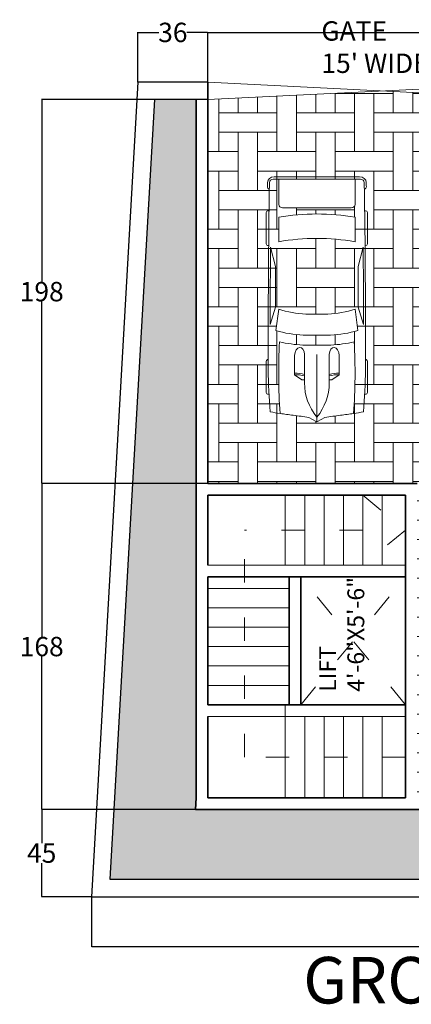
# Model space of a CAD drawing. Units: inches. Extents: x 377 to 1481, y 110 to 618.
# Tile 1 of 3: x 377 to 579, y 110 to 618. Entities that reach past the tile are written whole.
import ezdxf

# ---------------------------------------------------------------- set-up
doc = ezdxf.new("R2010")
doc.units = ezdxf.units.IN
doc.header["$MEASUREMENT"] = 0
doc.linetypes.add('ACAD_ISO03W100', pattern=[30, 12, -18])
for name, color, linetype, lineweight in [('A-ANNO-DIMS', 2, 'Continuous', 18), ('A-ANNO-TEXT', 7, 'Continuous', 18), ('A-ANNO-TITL', 7, 'Continuous', 35), ('A-AREA-IDEN', 7, 'Continuous', 18), ('A-EQPM-VEHI', 8, 'Continuous', 13), ('A-FLOR-EVTR-SYMB', 7, 'ACAD_ISO03W100', 13), ('A-FLOR-STRS', 7, 'Continuous', 20), ('A-FLOR-STRS-PATH', 7, 'ACAD_ISO03W100', 13), ('A-WALL', 7, 'Continuous', 35), ('C-PROP', 7, 'Continuous', 25), ('L-SITE-GATE', 3, 'Continuous', 18)]:
    doc.layers.add(name, color=color, linetype=linetype, lineweight=lineweight)
doc.layers.add('A-FLOR-PATT', color=252, linetype='Continuous', lineweight=13, true_color=0x939598)
doc.layers.add('L-PLNT-PATT', color=85, linetype='Continuous', lineweight=13, true_color=0x58ba48)
doc.styles.get("Standard").update_dxf_attribs({"font": 'arial.ttf'})
doc.dimstyles.get("Standard").update_dxf_attribs({"dimtxt": 10, "dimasz": 0.18, "dimexe": 0.18, "dimexo": 0.0625, "dimgap": 0.09, "dimtad": 0, "dimtih": 1, "dimtoh": 1, "dimdec": 0, "dimzin": 0, "dimdsep": 46, "dimlunit": 3, "dimtxsty": 'Standard', "dimcen": 0.09, "dimadec": 0, "dimazin": 0, "dimtfac": 1, "dimtdec": 0, "dimtofl": 0, "dimtmove": 0, "dimatfit": 3, "dimfxl": 1, "dimtolj": 1, "dimtzin": 0, "dimarcsym": 0})

# ---------------------------------------------------------------- blocks, each defined once
blk = doc.blocks.new('*U11')
for p, q in [((46.55368679439944, 38.88847654282876), (22.35054758993934, 38.88847654282876)), ((136.6978032355602, 38.88847654282876), (160.90094244002, 38.88847654282867)), ((21.10406751471477, 37.40863046792069), (21.10406751471477, 36.83230215753705)), ((47.80016686962392, 37.39011648242055), (47.80016686962392, 37.40863046792069)), ((70.0302824853563, 31.53613089391356), (86.40615155322342, 29.35124891408057)), ((87.98532186932616, 31.87120872459877), (74.75900729854769, 35.92175679182955)), ((134.313356548143, 35.6043097713567), (119.2882629232503, 31.77757799177584)), ((135.4513231603356, 37.07354110333037), (135.4513231603356, 37.40863046792069)), ((162.1474225152445, 37.40863046792049), (162.1474225152445, 36.77402019194128)), ((186.4728846989705, -33.49860931502491), (186.4728846989718, 33.49860931502465)), ((188.3990091454065, -32.75868627757393), (188.3990091454077, 32.75868627757058)), ((138.4228833961707, 29.35124891408074), (157.2465674415997, 29.35124891408074)), ((164.515393597658, 26.39155676426461), (164.5153935976578, -26.39155676426503)), ((186.4728846989718, 29.35124891408083), (167.0083537481071, 29.35124891408083)), ((32.26591480791686, 11.62530558863241), (36.12873726252356, 17.16961494239206)), ((36.12873726252356, 17.16961494239206), (50.93891189819171, 17.16961494239206)), ((29.77279020470884, 9.505833383620029), (51.68362801571248, 9.505833383620029)), ((32.12291633764599, 9.505833383620029), (32.12291633764599, 11.15369945057711)), ((58.9167604809788, -10.77488335095668), (58.9167604809788, 10.77488335095617)), ((66.55009204259746, -10.5288681329018), (66.55009204259746, 10.52886813290129)), ((82.73706193978568, 8.496039918672748), (82.73706193978568, -8.49603991867258)), ((186.4728846989718, -10.5288681329018), (186.4728846989718, 10.52886813290129)), ((3.266462181856987, 6.128290093440767), (0.1022408397004821, 0.4060708604429806)), ((-4.43e-14, -2.558e-13), (51.68362801571248, -2.558e-13)), ((0.1022408397004821, -0.4060708604432933), (3.266462181856987, -6.128290093441194)), ((29.77279020470884, -9.50583338362054), (51.68362801571248, -9.50583338362054)), ((32.12291633764599, -9.50583338362054), (32.12291633764599, -11.15369945057762)), ((32.26591480791686, -11.62530558863292), (36.12873726252356, -17.16961494239257)), ((36.12873726252356, -17.16961494239257), (50.93891189819171, -17.16961494239257)), ((86.40615155322318, -29.35124891408145), (70.03028248535594, -31.53613089391442)), ((157.2465674415997, -29.35124891408117), (138.4228833961707, -29.35124891408126)), ((167.008353748107, -29.35124891408126), (186.4728846989707, -29.35124891408108)), ((21.10406751471477, -37.4086304679212), (21.10406751471477, -36.83230215753756)), ((47.80016686962392, -37.39011648242107), (47.80016686962392, -37.4086304679212)), ((87.98532186932607, -31.87120872459903), (74.7590072985476, -35.92175679182964)), ((134.3133565481428, -35.60430977135721), (119.2882629232503, -31.77757799177618)), ((135.4513231603355, -37.07354110333088), (135.4513231603355, -37.4086304679212)), ((162.1474225152445, -37.408630467921), (162.1474225152445, -36.77402019194179)), ((46.55368679439944, -38.88847654282927), (22.35054758993934, -38.88847654282927)), ((136.6978032355602, -38.88847654282927), (160.9009424400199, -38.88847654282918))]:
    blk.add_line(p, q)
for centre, major_axis, ratio, start_param, end_param in [((22.35054758993934, 37.40863046792072), (2.08e-14, -1.479846074908118), 0.842303869543976, 3.141592653589776, 4.712388980384677), ((46.55368679439944, 37.40863046792072), (2.2e-14, 1.479846074908118), 0.8423038695439758, -1.570796326794884, 1.73e-14), ((136.6978032355602, 37.40863046792072), (2.357e-13, -1.479846074908118), 0.842303869543976, 3.141592653589603, 4.712388980384554), ((160.90094244002, 37.40863046792052), (5.59e-14, 1.479846074908118), 0.842303869543976, -1.570796326794865, 4.44e-14), ((180.6280394947615, 35.8381667808375), (7.4e-14, 2.219769112362114), 0.8423038695439693, -0.0130174256259048, 1.249894140392862), ((64.48199294754608, -10556.35759891604), (1.349839377e-06, 10595.3130398087), 0.8423038681351469, -0.0133969484821159, -0.0130174254969711), ((183.9799245485216, 32.75868627756583), (8.56e-14, -5.246425615115243), 0.8423038695439737, 1.570796326795794, 3.128195704978164), ((266.0300214172791, -27.52442688366631), (1.966072e-10, 313.3077612809058), 0.8423038695435284, 1.367075990158062, 1.391760499156098), ((41.19115208863305, -490.8631038926156), (1.294e-13, 528.2339998381949), 0.8423038695439741, 0.0028100083536837, 0.0755983031096952), ((64.48199294511879, -10555.61767587835), (1.907644e-10, 10593.02630634627), 0.842303869543847, -0.0133969486112073, 0.0027970409639888), ((135.2911776514449, 5.387441675478555), (2.2715e-12, 81.77258453065997), 0.8423038695439563, 1.245306111696802, 1.507880129813836), ((64.4819929449925, -10555.61767590795), (1.9177683e-09, -10591.54646030096), 0.8423038695482963, 3.133765086725325, 3.140440689641252), ((95.78879860270445, -3666.353346297651), (1.949864e-10, -3698.236159209632), 0.8423038695446962, 3.134048706297306, 3.14409775411291), ((183.9799245485226, 33.49860931502124), (3e-16, -2.959692149816168), 0.8423038695439952, 1.570796326796048, 3.128195704978389), ((259.1750197310735, -27.52442688366614), (1.506617e-10, -305.3028914627677), 0.8423038695443789, 4.528606069860317, 4.561837674556238), ((37.47375371777758, -593.9621830607928), (6.21e-14, -623.32820996736), 0.8423038695439826, 3.09604606856106, 3.200911180495224), ((134.4003789125686, 5.387441675477674), (4.276e-13, -89.7774543484738), 0.84230386954398, 4.44948196380473, 4.652344057257214), ((149.595361812917, 2.799442537139299), (8.561e-13, -79.57966406425402), 0.842303869543983, 4.372215489277867, 4.640744122441986), ((17.08207736189386, -1.421e-13), (6.87e-14, 147.0179238898305), 0.8423038695439764, 4.511394369635731, 4.913383591133647), ((35.90576140732288, -1.421e-13), (6.87e-14, 147.0179238898305), 0.8423038695439764, 4.511394369635731, 4.913383591133647), ((167.0083537481071, 26.39155676426464), (1.394e-13, 2.959692149816236), 0.842303869543976, 5.55e-14, 1.57079632679492), ((-204.4946649195746, 52.39684969293512), (4.12053e-11, -250.9602162198571), 0.8423038695441164, 1.385369446298923, 1.434372047871027), ((13.03653510440275, 17.00972444508943), (1.2303e-12, 27.41599049210566), 0.8423038695439277, 4.435146050259648, 4.718221029521873), ((14.20086229321332, 17.00972444508943), (1.2303e-12, 27.41599049210566), 0.8423038695439277, 4.435146050259648, 4.718221029521873), ((50.7902773840875, 13.33772416300607), (6.340077547122382, -0.356608581037027), 0.6038335755719145, -1.39555193967809, 1.581314658479915), ((29.77279020470884, -46.66302566589627), (5.12e-14, 56.16885904951626), 0.842303869543976, 7e-16, 0.5903187773915901), ((32.74615637525823, 11.15369945057713), (1.313e-13, 0.7399230374541176), 0.8423038695439091, 0.8797135699495516, 1.570796326795045), ((0.6232400376122422, -1.421e-13), (1e-16, -0.7399230374541245), 0.842303869543842, 4.131459131953847, 5.293318828815531), ((-204.4946649195746, -52.39684969293552), (4.02945e-11, 250.9602162198562), 0.8423038695441192, -1.43437204787103, -1.385369446298926), ((29.77279020470884, 46.66302566589578), (4.004e-13, 56.16885904951626), 0.8423038695439734, 2.55127387619821, 3.141592653589801), ((32.74615637525823, -11.1536994505777), (1.3e-13, -0.7399230374541176), 0.8423038695439093, 4.712388980384541, 5.403471737230034), ((13.03653510440275, -17.00972444508983), (1.2568e-12, -27.41599049210552), 0.8423038695439318, 1.564964277657711, 1.848039256919935), ((14.20086229321332, -17.00972444508983), (1.2568e-12, -27.41599049210552), 0.8423038695439318, 1.564964277657711, 1.848039256919935), ((134.4003789125684, -5.387441675478584), (4.2949e-12, -89.77745434847827), 0.8423038695439354, -1.510751403667474, -1.307889310215002), ((135.2911776514465, -5.387441675480715), (3.2038e-12, -81.77258453066244), 0.8423038695439492, -1.50788012981387, -1.245306111696839), ((149.5953618129329, -2.799442537137565), (4.0897e-12, -79.57966406427697), 0.8423038695439419, -1.499151468852248, -1.230622835688196), ((259.1750197310694, 27.52442688365929), (1.08535e-11, 305.3028914629043), 0.8423038695439974, 1.721347632622872, 1.754579237318777), ((266.0300214172791, 27.52442688366566), (8.75241e-11, 313.3077612806533), 0.8423038695441819, 1.749832154434603, 1.774516663432659), ((37.47375371777847, 593.9621830607904), (1.1693e-12, -623.3282099673584), 0.8423038695439528, -0.0593185269054384, 0.0455465850287298), ((167.008353748107, -26.39155676426503), (1.02e-14, -2.959692149816192), 0.8423038695439885, 4.712388980384686, 6.283185307179581), ((41.19115208863322, 490.8631038926152), (1.37757e-11, -528.2339998381949), 0.8423038695440652, -0.0755983031097181, -0.0028100083537155), ((22.35054758993934, -37.40863046792117), (2.2e-14, 1.479846074908118), 0.8423038695439758, 1.570796326794908, 3.14159265358981), ((64.48199294495228, 10555.61767590795), (6.117947e-10, 10593.02630637587), 0.8423038695458146, 3.138795612625926, 3.154989602201039), ((46.55368679439944, -37.40863046792117), (2.08e-14, -1.479846074908118), 0.842303869543976, -1.69e-14, 1.570796326794884), ((64.48199294503607, 10555.61767590793), (1.6049794e-09, -10591.54646030094), 0.8423038695397146, 0.0011519639481523, 0.0078275668641468), ((95.78879860271888, 3666.35334629765), (1.637818e-10, -3698.236159209629), 0.8423038695447546, -0.0025051005232382, 0.007543947292366), ((136.6978032355602, -37.40863046792109), (1.56e-14, -1.479846074908162), 0.8423038695440105, -1.570796326794875, -1.27e-14), ((160.9009424400199, -37.408630467921), (1.969e-13, 1.479846074908162), 0.8423038695440109, 3.141592653589951, 4.712388980384771), ((180.6280394947581, -35.83816678083949), (2.274e-13, -2.219769112363032), 0.8423038695439803, -1.249894138785958, 0.0130174256254374), ((183.9799245485216, -33.4986093150211), (9.3e-15, 2.959692149816141), 0.8423038695439732, 3.154989602201626, 4.71238898038339), ((183.9799245485177, -32.7586862775633), (2.428e-13, -5.246425615118353), 0.8423038695439808, 0.0133969486110846, 1.570796326792831), ((64.48199294197605, 10556.3575989598), (9.365289701e-07, 10595.31303985772), 0.8423038705260315, 3.154610079306566, 3.154989602290631)]:
    blk.add_ellipse(centre, major_axis=major_axis, ratio=ratio, start_param=start_param, end_param=end_param)
at = {"extrusion": (0, 0, -1)}
blk.add_ellipse((50.7902773840875, -13.33772416300655), major_axis=(6.340077547122382, 0.3566085810370246), ratio=0.6038335755719145, start_param=-1.39555193967809, end_param=1.581314658479915, dxfattribs=at)
blk = doc.blocks.new('STAIR-RETURN-3FLIGHT')
for p, q in [((40.00033022156276, 120.0003977439995), (40.00033022156265, 156.0003977439995)), ((50.00033022156276, 120.0003977439996), (50.00033022156265, 156.0003977439995)), ((60.00033022156276, 120.0003977439996), (60.00033022156265, 156.0003977439996)), ((70.00033022156276, 120.0003977439997), (70.00033022156265, 156.0003977439996)), ((80.00033022156276, 120.0003977439997), (80.00033022156263, 156.0003977439997)), ((90.00033022156276, 120.0003977439998), (90.00033022156263, 156.0003977439997)), ((102.0003302215626, 120.0003977439996), (102.0003302215626, 156.0003977439995)), ((0.0003302215625922, 120.0003977439995), (102.0003302215626, 120.0003977439996)), ((0.0003302215626491, 108.0003977439995), (42.00033022156264, 108.0003977439995)), ((0.0003302215626491, 98.00039774399956), (42.00033022156264, 98.00039774399956)), ((0.0003302215626491, 88.00039774399953), (42.00033022156264, 88.00039774399953)), ((0.0003302215626491, 78.00039774399954), (42.00033022156264, 78.00039774399954)), ((0.0003302215626491, 68.00039774399954), (42.00033022156264, 68.00039774399954)), ((0.0003302215626491, 58.00039774399954), (42.00033022156264, 58.00039774399954)), ((40.00033022156265, 0.0003977439995992), (40.00033022156253, 48.00039774399954)), ((0.0003302215626491, 42.00039774399954), (102.0003302215626, 42.0003977439996)), ((50.00033022156265, 0.0003977439996277), (50.00033022156253, 42.00039774399954)), ((60.00033022156265, 0.0003977439996561), (60.00033022156253, 42.00039774399954)), ((70.00033022156265, 0.0003977439996845), (70.00033022156254, 42.00039774399954)), ((80.00033022156263, 0.0003977439997129), (80.00033022156254, 42.00039774399954)), ((90.00033022156263, 0.0003977439997414), (90.00033022156254, 42.00039774399954)), ((102.0003302215626, 0.0003977439995992), (102.0003302215626, 42.0003977439996))]:
    blk.add_line(p, q)
blk = doc.blocks.new('STAIR-PATH-UP')
for p, q in [((60.98933022156273, 117.0003977439996), (60.98933022156263, 135.0003977439995)), ((60.98933022156263, 135.0003977439995), (82.98933022156262, 117.0003977439996)), ((0.0003307549570195, 0.0003977439995992), (0.0003307549570195, 117.0003977439995)), ((60.98933022156273, 117.0003977439996), (0.0003307549569627, 117.0003977439996)), ((60.98933022156273, 119.0371309909091), (60.98933022156273, 99.00039774399978)), ((82.98933022156262, 117.0003977439996), (60.98933022156273, 99.00039774399978)), ((82.98933022156262, 0.0003977439995992), (0.0003307549570195, 0.0003977439995992))]:
    blk.add_line(p, q)
blk = doc.blocks.new('LIFT-SHAFT-MARK')
for p, q in [((0.0003302215626491, 0.0003977439995424), (54.00033022156264, 66.00039774399959)), ((54.00033022156264, 0.0003977439995992), (0.0003302215626491, 66.00039774399959))]:
    blk.add_line(p, q)
blk = doc.blocks.new('*D27')
at = {"layer": 'A-ANNO-DIMS', "color": 0, "lineweight": -2, "transparency": 16777216}
for p, q in [((414.320847, 165.776898), (414.320847, 140.009398)), ((882.3208469999998, 165.776898), (882.3208469999998, 140.009398)), ((414.500847, 140.189398), (636.9723203969986, 140.189398)), ((882.1408469999999, 140.189398), (659.6693736030013, 140.189398))]:
    blk.add_line(p, q, dxfattribs=at)
at = {"layer": 'A-ANNO-DIMS', "color": 0, "lineweight": 100, "transparency": 16777216}
for points in [[(414.500847, 140.219398), (414.500847, 140.159398), (414.320847, 140.189398)], [(882.1408469999999, 140.219398), (882.1408469999999, 140.159398), (882.3208469999998, 140.189398)]]:
    blk.add_solid(points, dxfattribs=at)
at = {"layer": 'Defpoints', "color": 0, "lineweight": 100, "transparency": 16777216}
for p in [(414.320847, 165.839398), (882.3208469999998, 165.839398), (882.3208469999998, 140.189398)]:
    blk.add_point(p, dxfattribs=at)
at = {"layer": 'A-ANNO-DIMS', "color": 0, "transparency": 16777216, "insert": (648.320847, 140.189398), "char_height": 10, "attachment_point": 5}
blk.add_mtext('\\A1;468', dxfattribs=at)
blk = doc.blocks.new('*D29')
at = {"layer": 'A-ANNO-DIMS', "color": 0, "lineweight": -2, "transparency": 16777216}
for p, q in [((438.320847, 585.901898), (438.320847, 611.6693979999999)), ((438.500847, 611.489398), (449.0740632612551, 611.489398)), ((474.1383299999999, 611.489398), (463.5651137387449, 611.489398)), ((474.31833, 585.901898), (474.31833, 611.6693979999999))]:
    blk.add_line(p, q, dxfattribs=at)
at = {"layer": 'A-ANNO-DIMS', "color": 0, "lineweight": 100, "transparency": 16777216}
for points in [[(438.500847, 611.519398), (438.500847, 611.4593980000001), (438.320847, 611.489398)], [(474.1383299999999, 611.519398), (474.1383299999999, 611.4593980000001), (474.31833, 611.489398)]]:
    blk.add_solid(points, dxfattribs=at)
at = {"layer": 'Defpoints', "color": 0, "lineweight": 100, "transparency": 16777216}
for p in [(474.31833, 611.489398), (438.320847, 585.8393979999998), (474.31833, 585.8393979999998)]:
    blk.add_point(p, dxfattribs=at)
at = {"layer": 'A-ANNO-DIMS', "color": 0, "transparency": 16777216, "insert": (456.3195884999999, 611.489398), "char_height": 10, "attachment_point": 5}
blk.add_mtext('\\A1;36', dxfattribs=at)
blk = doc.blocks.new('*D30')
at = {"layer": 'A-ANNO-DIMS', "color": 0, "lineweight": -2, "transparency": 16777216}
for p, q in [((474.31833, 576.9018979999998), (474.31833, 611.6693979999999)), ((474.49833, 611.489398), (641.6859322926329, 611.489398)), ((831.1408469999999, 611.489398), (663.953244707367, 611.489398)), ((831.3208469999998, 576.9018979999998), (831.3208469999998, 611.6693979999999))]:
    blk.add_line(p, q, dxfattribs=at)
at = {"layer": 'A-ANNO-DIMS', "color": 0, "lineweight": 100, "transparency": 16777216}
for points in [[(474.49833, 611.519398), (474.49833, 611.4593980000001), (474.31833, 611.489398)], [(831.1408469999999, 611.519398), (831.1408469999999, 611.4593980000001), (831.3208469999998, 611.489398)]]:
    blk.add_solid(points, dxfattribs=at)
at = {"layer": 'Defpoints', "color": 0, "lineweight": 100, "transparency": 16777216}
for p in [(831.3208469999998, 611.489398), (474.31833, 576.8393979999998), (831.3208469999998, 576.8393979999998)]:
    blk.add_point(p, dxfattribs=at)
at = {"layer": 'A-ANNO-DIMS', "color": 0, "transparency": 16777216, "insert": (652.8195885, 611.489398), "char_height": 10, "attachment_point": 5}
blk.add_mtext('\\A1;357', dxfattribs=at)
blk = doc.blocks.new('*D32')
at = {"layer": 'A-ANNO-DIMS', "color": 0, "lineweight": -2, "transparency": 16777216}
for p, q in [((467.9129730000002, 210.8393980000001), (388.4908470000004, 210.8393980000001)), ((388.6708470000004, 210.6593980000001), (388.6708470000004, 193.5146640300137)), ((388.6708470000004, 166.019398), (388.6708470000004, 183.1641319699864)), ((414.2583470000002, 165.839398), (388.4908470000004, 165.839398))]:
    blk.add_line(p, q, dxfattribs=at)
at = {"layer": 'A-ANNO-DIMS', "color": 0, "lineweight": 100, "transparency": 16777216}
for points in [[(388.6408470000004, 210.6593980000001), (388.7008470000004, 210.6593980000001), (388.6708470000004, 210.8393980000001)], [(388.6408470000004, 166.019398), (388.7008470000004, 166.019398), (388.6708470000004, 165.839398)]]:
    blk.add_solid(points, dxfattribs=at)
at = {"layer": 'Defpoints', "color": 0, "lineweight": 100, "transparency": 16777216}
for p in [(388.6708470000004, 210.8393980000001), (467.9754730000002, 210.8393980000001), (414.3208470000002, 165.839398)]:
    blk.add_point(p, dxfattribs=at)
at = {"layer": 'A-ANNO-DIMS', "color": 0, "transparency": 16777216, "insert": (388.6708470000004, 188.3393979999999), "char_height": 10, "attachment_point": 5}
blk.add_mtext('\\A1;45', dxfattribs=at)
blk = doc.blocks.new('*D33')
at = {"layer": 'A-ANNO-DIMS', "color": 0, "lineweight": -2, "transparency": 16777216}
for p, q in [((474.2558300000002, 378.8393980000001), (388.4908470000004, 378.8393980000001)), ((388.6708470000004, 378.6593980000001), (388.6708470000004, 300.0351278772171)), ((388.6708470000004, 211.0193980000001), (388.6708470000004, 289.6436681227832)), ((467.9129730000002, 210.8393980000001), (388.4908470000004, 210.8393980000001))]:
    blk.add_line(p, q, dxfattribs=at)
at = {"layer": 'A-ANNO-DIMS', "color": 0, "lineweight": 100, "transparency": 16777216}
for points in [[(388.6408470000004, 378.6593980000001), (388.7008470000004, 378.6593980000001), (388.6708470000004, 378.8393980000001)], [(388.6408470000004, 211.0193980000001), (388.7008470000004, 211.0193980000001), (388.6708470000004, 210.8393980000001)]]:
    blk.add_solid(points, dxfattribs=at)
at = {"layer": 'Defpoints', "color": 0, "lineweight": 100, "transparency": 16777216}
for p in [(388.6708470000004, 378.8393980000001), (474.3183300000002, 378.8393980000001), (467.9754730000002, 210.8393980000001)]:
    blk.add_point(p, dxfattribs=at)
at = {"layer": 'A-ANNO-DIMS', "color": 0, "transparency": 16777216, "insert": (388.6708470000004, 294.839398), "char_height": 10, "attachment_point": 5}
blk.add_mtext('\\A1;168', dxfattribs=at)
blk = doc.blocks.new('*D34')
at = {"layer": 'A-ANNO-DIMS', "color": 0, "lineweight": -2, "transparency": 16777216}
for p, q in [((474.2558300000002, 576.8393980000001), (388.4908470000004, 576.8393980000001)), ((388.6708470000004, 576.6593980000002), (388.6708470000004, 483.035127877217)), ((388.6708470000005, 379.0193980000001), (388.6708470000004, 472.6436681227832)), ((474.2558300000002, 378.8393980000001), (388.4908470000005, 378.8393980000001))]:
    blk.add_line(p, q, dxfattribs=at)
at = {"layer": 'A-ANNO-DIMS', "color": 0, "lineweight": 100, "transparency": 16777216}
for points in [[(388.6408470000004, 576.6593980000002), (388.7008470000004, 576.6593980000002), (388.6708470000004, 576.8393980000001)], [(388.6408470000005, 379.0193980000001), (388.7008470000005, 379.0193980000001), (388.6708470000005, 378.8393980000001)]]:
    blk.add_solid(points, dxfattribs=at)
at = {"layer": 'Defpoints', "color": 0, "lineweight": 100, "transparency": 16777216}
for p in [(388.6708470000004, 576.8393980000001), (474.3183300000002, 576.8393980000001), (474.3183300000002, 378.8393980000001)]:
    blk.add_point(p, dxfattribs=at)
at = {"layer": 'A-ANNO-DIMS', "color": 0, "transparency": 16777216, "insert": (388.6708470000005, 477.8393979999999), "char_height": 10, "attachment_point": 5}
blk.add_mtext('\\A1;198', dxfattribs=at)

msp = doc.modelspace()

# ---------------------------------------------------------------- hatches: boundary and pattern name
at = {"layer": 'A-FLOR-PATT'}
h = msp.add_hatch(dxfattribs=at)
h.set_pattern_fill('±ÀÖ¯²ÄÁÏ', color=256, scale=20)
h.set_pattern_definition([(0, (0, 0), (20, 20), [30, -10]), (0, (0, 10), (20, 20), [30, -10]), (90, (10, 10), (-20, 20), [30, -10]), (90, (20, 10), (-20, 20), [30, -10])])
h.paths.add_polyline_path([(831.3208470620848, 576.8393977439996), (654.3183302215624, 576.8393977439996), (564.3183302215629, 581.3393977439996), (474.3183302215626, 576.8393977439996), (474.3183302215626, 378.8393977439996), (582.3183302215626, 378.8393977439995), (582.3183302215626, 216.8393977439996), (681.320847062085, 216.8393977439997), (681.3208470620849, 378.8393977439995), (793.3762999136519, 378.8393977439995), (793.3762999136519, 373.4477156717346, 0.4014527144963569), (827.7482731243409, 337.537585054926), (827.7482731243409, 373.4477156717346), (829.3208470620848, 373.4477156717346), (829.3208470620848, 378.8393977439996), (831.3208470620848, 378.8393977439995)])
h.paths.add_polyline_path([(655.1112320992189, 487.8017993641329), (655.1112320992189, 521.5563777088427), (655.1112320992189, 555.3233738998766, -0.3760864404517753), (659.767292319398, 558.8161256031975), (665.5887632688018, 558.8161256031975, -0.3333350785240507), (669.0813054040638, 555.3236063246482), (669.0813092134161, 555.3236063246482), (811.1104303504404, 555.3236063246482, -0.3333350785240531), (814.6029724857026, 558.8161256031975), (820.4244434351054, 558.8161256031975, -0.3760864404519927), (825.0805036552854, 555.3233738998733), (825.0805036552854, 521.5687955551666), (825.0805036552854, 487.8017993641362, -0.3760864404520696), (820.4244434351043, 484.3090476608121), (814.6029724857024, 484.3090476608121, -0.3333350785240366), (811.1104303504404, 487.8015669393615), (811.1104265410881, 487.8015669393615), (669.0813054040638, 487.8015669393615, -0.3333350785240358), (665.588763268802, 484.3090476608121), (659.7672923193994, 484.3090476608121, -0.3760864404518541)], flags=16)
h.paths.add_polyline_path([(659.7679244706181, 521.5563777088427), (659.7679244706181, 528.5476251891034), (708.6631943703085, 535.532663746202), (708.6631943703085, 555.3236063246482), (722.6332714845057, 546.01022158185), (778.5135799412946, 546.01022158185), (785.4986184983933, 555.3236063246482), (785.4986184983933, 521.5625866320047), (785.4986184983933, 487.8015669393614), (778.5135799412946, 497.1149516821596), (722.6332714845057, 497.1149516821596), (708.6631943703085, 487.8015669393615), (708.6631943703085, 507.5925095178076), (659.7679244706181, 514.5775480749062)], flags=0)
edge = h.paths.add_edge_path(flags=16)
edge.add_ellipse((512.141418614859, 584.5696558424829), major_axis=(-204.7255748268525, 9.67931e-11), ratio=0.8423038695443797, start_angle=100.2095389971704, end_angle=102.44462729347111, ccw=False)
edge.add_ellipse((565.7338664611478, 273.648778987746), major_axis=(168.2852536317261, 6.42065e-11), ratio=0.842303869543657, start_angle=99.25656600717964, end_angle=102.5549326441154)
edge.add_line((534.707768362197, 412.9662154153117), (530.5983486771285, 410.6938254662535))
edge.add_line((530.5983486771285, 410.6938254662535), (526.4889289920602, 412.9662154153116))
edge.add_ellipse((495.4628308931093, 273.648778987746), major_axis=(168.2852536315943, 6.1815e-11), ratio=0.8423038695442986, start_angle=77.44506735584166, end_angle=80.74343399277738)
edge.add_ellipse((549.0552787394023, 584.5696558424856), major_axis=(204.7255748269201, 3.28788e-11), ratio=0.8423038695441253, start_angle=257.5553727065455, end_angle=259.7904610028463, ccw=False)
edge.add_ellipse((928.8888750783977, 435.9044437085582), major_axis=(-417.9823698359099, 1.184e-13), ratio=0.842303869543927, start_angle=-2.1985405659551134, end_angle=2.8637146078376077, ccw=False)
edge.add_ellipse((526.9857163546047, 500.9000910277084), major_axis=(60.20166025916774, 4.181e-13), ratio=0.8423038695439812, start_angle=252.2800467772492, end_angle=265.917589308849)
edge.add_line((523.3730840320812, 450.283383470902), (537.8236133221772, 450.283383470902))
edge.add_ellipse((534.2109809996527, 500.9000910277083), major_axis=(60.201660259169, 1.2736e-12), ratio=0.8423038695439622, start_angle=-85.91758930885108, end_angle=-72.28004677725126)
edge.add_ellipse((132.3078222758608, 435.9044437085587), major_axis=(-417.9823698359087, 2.3459e-12), ratio=0.8423038695438743, start_angle=177.1362853921626, end_angle=182.1985405659555, ccw=False)
edge = h.paths.add_edge_path(flags=16)
edge.add_ellipse((534.2109809996541, 501.4974298966528), major_axis=(54.83387102201502, 2.4993e-12), ratio=0.8423038695439453, start_angle=-85.7225790369485, end_angle=-68.16504620329431, ccw=False)
edge.add_line((537.6586440135299, 455.4020319851987), (523.5380533407272, 455.4020319851987))
edge.add_ellipse((526.985716354604, 501.4974298966517), major_axis=(-54.8338710220135, 2.0245e-12), ratio=0.8423038695439498, start_angle=68.16504620329238, end_angle=85.72257903694663, ccw=False)
edge.add_line((509.4513084570433, 457.7357275014352), (510.9164148538646, 468.7168197280619))
edge.add_ellipse((528.721139195539, 511.0893217744386), major_axis=(53.3633742937202, 3.469e-13), ratio=0.8423038695439728, start_angle=247.2080851224096, end_angle=265.1299304028639)
edge.add_line((524.9011977337861, 466.2564549519428), (536.295499620471, 466.2564549519428))
edge.add_ellipse((532.4755581587168, 511.0893217744494), major_axis=(53.36337429373605, 3.8424e-12), ratio=0.8423038695439261, start_angle=-85.12993040286842, end_angle=-67.20808512241756)
edge.add_line((550.2802825003928, 468.7168197280617), (551.7453888972141, 457.735727501435))
edge = h.paths.add_edge_path(flags=0)
edge.add_line((542.111699473761, 444.9337137407289), (542.111699473761, 435.0025221262431))
edge.add_line((542.111699473761, 435.0025221262431), (538.2562464159993, 432.3163569622979))
edge.add_line((538.2562464159993, 432.3163569622979), (536.972632243019, 432.3163569622979))
edge.add_line((536.972632243019, 432.3163569622979), (536.972632243019, 430.7404435434111))
edge.add_ellipse((499.3077352576486, 430.740443543411), major_axis=(-37.66489698537048, 7.634e-13), ratio=0.8423038695439682, start_angle=150.5614304020218, end_angle=180.0000000000012, ccw=False)
edge.add_ellipse((561.8889620966085, 430.740443543411), major_axis=(37.66489698537043, 6.965e-13), ratio=0.8423038695439699, start_angle=179.9999999999989, end_angle=209.4385695979783, ccw=False)
edge.add_line((524.2240651112381, 430.7404435434107), (524.2240651112381, 432.3163569622979))
edge.add_line((524.2240651112381, 432.3163569622979), (522.940450938258, 432.3163569622979))
edge.add_line((522.940450938258, 432.3163569622979), (519.0849978804961, 435.0025221262431))
edge.add_line((519.0849978804961, 435.0025221262431), (519.0849978804961, 444.9337137407288))
edge.add_ellipse((521.6545314958671, 444.8340445689326), major_axis=(0.2391293983204887, 4.251437037044111), ratio=0.6038335755719065, start_angle=-73.65740804569998, end_angle=90.99798572497588, ccw=False)
edge.add_line((524.2240651112381, 445.4330946490179), (524.2240651112381, 430.7404435434109))
edge.add_ellipse((561.8889620966085, 430.740443543411), major_axis=(37.66489698537043, 6.965e-13), ratio=0.8423038695439699, start_angle=179.9999999999989, end_angle=209.4385695979783)
edge.add_ellipse((499.3077352576486, 430.740443543411), major_axis=(-37.66489698537048, 7.634e-13), ratio=0.8423038695439682, start_angle=150.5614304020218, end_angle=180.0000000000011)
edge.add_line((536.972632243019, 430.7404435434112), (536.972632243019, 445.4330946490189))
edge.add_ellipse((539.5421658583901, 444.8340445689326), major_axis=(-0.2391293983215679, 4.251437037044156), ratio=0.6038335755718898, start_angle=269.00201427500974, end_angle=433.6574080456862, ccw=False)
edge = h.paths.add_edge_path(flags=16)
edge.add_ellipse((530.5983486771285, 422.2304898077624), major_axis=(-98.58514223035905, 4.876e-13), ratio=0.8423038695439689, start_angle=256.4018653097696, end_angle=283.5981346902308)
edge.add_line((510.9164148538645, 503.5974436099374), (510.9164148538645, 516.2199560207953))
edge.add_ellipse((530.5983486771285, 434.8530022186204), major_axis=(98.5851422303597, 9.36e-14), ratio=0.8423038695439631, start_angle=76.40186530976939, end_angle=103.5981346902305, ccw=False)
edge.add_line((550.2802825003926, 516.2199560207953), (550.2802825003928, 503.5974436099373))
edge = h.paths.add_edge_path(flags=16)
edge.add_ellipse((548.2956151630524, 522.7658727769762), major_axis=(1.98466733734017, 1.09e-13), ratio=0.8423038695439435, start_angle=269.9999999999969, end_angle=359.9999999999969, ccw=False)
edge.add_line((548.2956151630524, 521.094179798977), (512.9010821912045, 521.0941797989772))
edge.add_ellipse((512.9010821912045, 522.7658727769762), major_axis=(1.984667337340112, 5.52e-14), ratio=0.8423038695439679, start_angle=179.9999999999985, end_angle=269.9999999999984, ccw=False)
edge.add_line((510.9164148538645, 522.7658727769762), (510.9164148538645, 535.8181149898111))
edge.add_line((510.9164148538645, 535.8181149898111), (550.2802825003924, 535.8181149898103))
edge.add_line((550.2802825003924, 535.8181149898103), (550.2802825003926, 522.7658727769762))
h.paths.add_polyline_path([(592.3367361683343, 230.4436529032155), (592.3367361683343, 242.646927118768), (582.0331891014856, 242.646927118768), (582.0331891014856, 230.4436529032155)], flags=24)
at = {"layer": 'L-PLNT-PATT'}
h = msp.add_hatch(color=256, dxfattribs=at)
h.dxf.hatch_style = 1
h.paths.add_polyline_path([(468.3183302215627, 576.8393977439996), (446.8212432498917, 576.8393977439996), (423.8498146784631, 174.8393977439996), (873.320847062085, 174.8393977439996), (873.3208470620846, 576.8393977439996), (837.3208470620848, 576.8393977439996), (837.3208470620848, 210.8393977439996), (467.9754730787054, 210.8393977439996), (468.3183302215626, 216.8393977440005)])

# ---------------------------------------------------------------- linework, layer by layer
at = {"layer": 'A-WALL'}
for p, q in [((474.3183302215626, 378.8393977439995), (474.3183302215626, 585.8393977439996)), ((468.3183302215626, 216.8393977439996), (468.3183302215627, 576.8393977439996)), ((474.3183302215626, 378.8393977439996), (582.3183302215626, 378.8393977439995)), ((474.3183302215626, 372.8393977439996), (576.3183302215627, 372.8393977439996)), ((474.3183302215626, 336.8393977439995), (474.3183302215626, 372.8393977439995)), ((576.3183302215626, 216.8393977439996), (576.3183302215627, 372.8393977439996)), ((474.3183302215626, 330.8393977439995), (576.3183302215626, 330.8393977439996)), ((474.3183302215626, 264.8393977439996), (474.3183302215626, 330.8393977439995)), ((516.3183302215626, 264.8393977439996), (516.3183302215626, 330.8393977439995)), ((522.3183302215626, 264.8393977439996), (522.3183302215626, 330.8393977439995)), ((474.3183302215626, 264.8393977439996), (576.3183302215626, 264.8393977439996)), ((474.3183302215626, 216.8393977439996), (474.3183302215624, 258.8393977439996)), ((468.3183302215625, 216.8393977439996), (467.9754730787054, 210.8393977439996)), ((474.3183302215626, 216.8393977439996), (576.3183302215626, 216.8393977439996)), ((467.9754730787053, 210.8393977439996), (837.3208470620848, 210.8393977439996))]:
    msp.add_line(p, q, dxfattribs=at)
at = {"layer": 'C-PROP'}
for p, q in [((438.3208470620847, 585.8393977439996), (414.3208470620847, 165.8393977439996)), ((474.3183302215626, 585.8393977439996), (438.3208470620847, 585.8393977439996)), ((446.8212432498917, 576.8393977439996), (423.8498146784631, 174.8393977439996)), ((474.3183302215626, 576.8393977439996), (446.8212432498918, 576.8393977439995)), ((423.8498146784632, 174.8393977439996), (873.3208470620848, 174.8393977439996)), ((414.3208470620847, 165.8393977439996), (882.3208470620848, 165.8393977439996))]:
    msp.add_line(p, q, dxfattribs=at)
at = {"layer": 'L-SITE-GATE'}
for p, q in [((654.3183302215626, 576.8393977439996), (474.3183302215626, 585.8393977439996)), ((474.3183302215626, 576.8393977439996), (654.3183302215626, 585.8393977439996))]:
    msp.add_line(p, q, dxfattribs=at)

# ---------------------------------------------------------------- block references
at = {"layer": 'A-EQPM-VEHI', "xscale": 0.6705654631896043, "yscale": 0.6705654631896043, "zscale": 0.6705654631896043, "rotation": 90}
msp.add_blockref('*U11', (530.5983486771285, 410.7758386893435), dxfattribs=at)
at = {"layer": 'A-FLOR-EVTR-SYMB'}
msp.add_blockref('LIFT-SHAFT-MARK', (522.318, 264.839), dxfattribs=at)
at = {"layer": 'A-FLOR-STRS'}
msp.add_blockref('STAIR-RETURN-3FLIGHT', (474.3179999999999, 216.839), dxfattribs=at)
at = {"layer": 'A-FLOR-STRS-PATH'}
msp.add_blockref('STAIR-PATH-UP', (493.329, 237.839), dxfattribs=at)

# ---------------------------------------------------------------- texts
at = {"layer": 'A-ANNO-TEXT', "insert": (532.9243151521782, 617.2521118760563), "char_height": 10, "attachment_point": 1}
msp.add_mtext_dynamic_manual_height_columns("GATE\\P15' WIDE", width=70.11836276200438, gutter_width=1, heights=[0], dxfattribs=at)
at = {"layer": 'A-ANNO-TITL', "insert": (523.5625681240535, 134.8117828229256), "char_height": 24, "attachment_point": 1}
msp.add_mtext_dynamic_manual_height_columns('{\\fTimes New Roman|b0|i0|c0|p18;GROUND FLOOR}', width=313.0421048124909, gutter_width=1, heights=[94.3060019033042], dxfattribs=at)
at = {"layer": 'A-AREA-IDEN', "insert": (531.8493849437857, 271.5050266116145), "char_height": 8.699522687298312, "attachment_point": 1, "rotation": 90}
msp.add_mtext_dynamic_manual_height_columns('LIFT\\P4\'-6"X5\'-6"', width=60.99962876442702, gutter_width=0.8699522687298312, heights=[0], dxfattribs=at)

# ---------------------------------------------------------------- dimensions: what is measured, and where the dimension line sits
at = {"layer": 'A-ANNO-DIMS'}
for base, p1, p2, picture, middle in [((474.31833, 611.489398), (438.320847, 585.8393979999998), (474.31833, 585.8393979999998), '*D29', (456.3195884999999, 611.489398)), ((831.3208469999998, 611.489398), (474.31833, 576.8393979999998), (831.3208469999998, 576.8393979999998), '*D30', (652.8195885, 611.489398)), ((882.3208469999998, 140.189398), (414.320847, 165.839398), (882.3208469999998, 165.839398), '*D27', (648.320847, 140.189398))]:
    dim = msp.add_linear_dim(base=base, p1=p1, p2=p2, dimstyle='Standard', override={"dimdec": 0, "dimlfac": 1, "dimrnd": 0, "dimzin": 0, "dimdsep": 46, "dimlunit": 2}, dxfattribs=at)
    dim.commit()
    dim.dimension.update_dxf_attribs({"geometry": picture, "text_midpoint": middle})
for base, p1, p2, picture, middle in [((388.6708470000004, 576.8393980000001), (474.31833, 378.839398), (474.31833, 576.8393979999998), '*D34', (388.6708470000005, 477.8393979999999)), ((388.6708470000004, 378.8393980000001), (467.9754729999999, 210.839398), (474.31833, 378.839398), '*D33', (388.6708470000004, 294.839398)), ((388.6708470000004, 210.8393980000001), (414.320847, 165.839398), (467.9754729999999, 210.839398), '*D32', (388.6708470000004, 188.3393979999999))]:
    dim = msp.add_linear_dim(base=base, p1=p1, p2=p2, angle=90, dimstyle='Standard', override={"dimdec": 0, "dimlfac": 1, "dimrnd": 0, "dimzin": 0, "dimdsep": 46, "dimlunit": 2}, dxfattribs=at)
    dim.commit()
    dim.dimension.update_dxf_attribs({"geometry": picture, "text_midpoint": middle})

doc.saveas('drawing.dxf')
